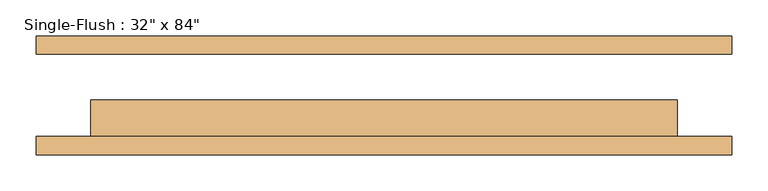
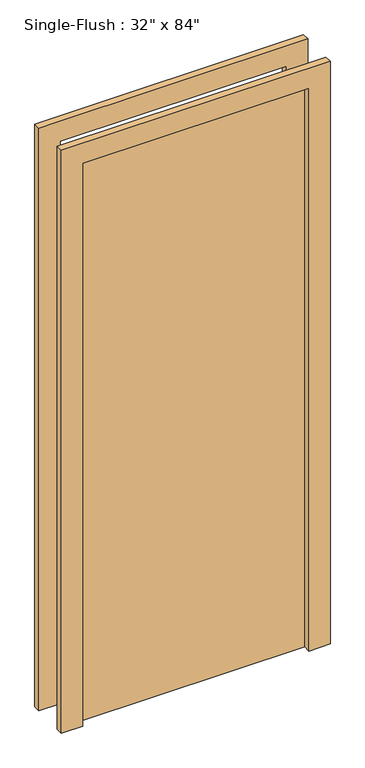
"""IFC4 building model written with IfcOpenShell, lengths in millimetres: door geometry."""

from ifc_helpers import new_model, si_unit, frame, origin, origin_with_axes, place, context, project, spatial, polyline, outline, extrude, source, transform, mapped, element, save


def door_38851409(model_context):
    return source(origin(), model_context, "Body", "SweptSolid", [
        extrude(outline(polyline([(2209.8, -482.6), (0.0, -482.6), (0.0, -406.4), (2133.6, -406.4), (2133.6, 406.4), (0.0, 406.4), (0.0, 482.6), (2209.8, 482.6), (2209.8, -482.6)])), frame((0.0, -82.55, 0.0), z_axis=(0.0, 1.0, 0.0), x_axis=(0.0, 0.0, 1.0)), (0.0, 0.0, 1.0), 25.4),
        extrude(outline(polyline([(2209.8, 482.6), (2209.8, -482.6), (0.0, -482.6), (0.0, -406.4), (2133.6, -406.4), (2133.6, 406.4), (0.0, 406.4), (0.0, 482.6), (2209.8, 482.6)])), frame((0.0, 57.15, 0.0), z_axis=(0.0, 1.0, 0.0), x_axis=(0.0, 0.0, 1.0)), (0.0, 0.0, 1.0), 25.4),
        extrude(outline(polyline([(406.4, -6.35), (406.4, -57.15), (-406.4, -57.15), (-406.4, -6.35), (406.4, -6.35)])), origin_with_axes(), (0.0, 0.0, 1.0), 2133.6),
    ])


if __name__ == "__main__":
    model = new_model("IFC4")
    model_context = context("Model", 3, world=origin())
    ifc_project = project(units=[si_unit("LENGTHUNIT", "METRE", prefix="MILLI")], contexts=[model_context])
    site = spatial("IfcSite", under=ifc_project)
    building = spatial("IfcBuilding", under=site)
    placement = place(None, origin())
    door_shape = door_38851409(model_context)
    element("IfcDoor", 1, ObjectType="Single-Flush : 32\" x 84\"", at=placement, inside=building, context=model_context, shape_type="MappedRepresentation", body=[
        mapped(door_shape, transform((0.0, 0.0, 0.0), x_axis=(1.0, 0.0, 0.0), y_axis=(0.0, 1.0, 0.0), z_axis=(0.0, 0.0, 1.0))),
    ])
    save(model, "model.ifc")

# Revit data of these elements
# Type "Single-Flush : 32\" x 84\""
#   Type Mark = "3"
#   Construction Type Id = "MDOOR"
#   Assembly Code = "C1020"
#   Analytic Construction = "Metal"
#   Thickness = 0' - 2"
#   Heat Transfer Coefficient (U) = 0.651978 BTU/(h·ft²·°F)
#   Height = 7' - 0"
#   Trim Projection Ext = 0' - 1"
#   Trim Projection Int = 0' - 1"
#   Trim Width = 0' - 3"
#   Width = 2' - 8"
#   Define Thermal Properties by = 1
#   Define Thermal Properties by = 1
#   Door Material = Door - Panel
#   Frame Material = Door - Frame
#   Visual Light Transmittance = 0
#   Solar Heat Gain Coefficient = 0
#   Function = (empty or 0)
#   Wall Closure = (empty or 0)
# Element 1 (IfcDoor, "Single-Flush : 32\" x 84\"")
#   Materials on its faces: "Door - Frame", "Door - Panel"
# Materials
#   "Door - Panel": class "Wood", colour RGB 210 159 95, transparency 0, Cost = 0
#   "Door - Frame": colour RGB 118 70 51, transparency 0, Cost = 0
